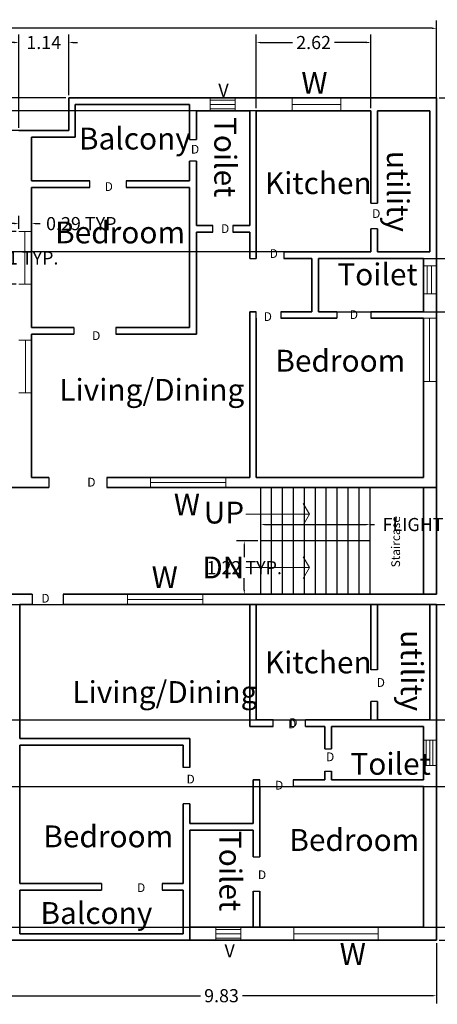
# Model space of a CAD drawing. Units: metres. Extents: x 11 to 49.6, y -23.3 to -0.8.
# Tile 4 of 5: x 25.8 to 35.3, y -23.3 to -0.8. Entities that reach past the tile are written whole.
import ezdxf

# ---------------------------------------------------------------- set-up
doc = ezdxf.new("R2010")
doc.units = ezdxf.units.M
doc.header["$MEASUREMENT"] = 0
for name, color, linetype, lineweight in [('A-ANNO-DIMS', 2, 'Continuous', 18), ('A-ANNO-IDEN', 3, 'Continuous', 18), ('A-ANNO-SYMB', 3, 'Continuous', 18), ('A-AREA-IDEN', 7, 'Continuous', 18), ('A-DOOR', 3, 'Continuous', 25), ('A-FLOR-STRS', 7, 'Continuous', 25), ('A-GLAZ', 4, 'Continuous', 18), ('A-GLAZ-VENT', 4, 'Continuous', 18), ('A-WALL', 7, 'Continuous', 35)]:
    doc.layers.add(name, color=color, linetype=linetype, lineweight=lineweight)
doc.styles.get("Standard").update_dxf_attribs({"font": 'arial.ttf'})
doc.dimstyles.get("Standard").update_dxf_attribs({"dimtxt": 0.3, "dimasz": 0.1, "dimexe": 0.18, "dimexo": 0.0625, "dimgap": 0.09, "dimtad": 0, "dimtih": 1, "dimtoh": 1, "dimzin": 0, "dimdsep": 46, "dimtxsty": 'Standard', "dimcen": 0.09, "dimadec": 0, "dimazin": 0, "dimtfac": 1, "dimtofl": 0, "dimtmove": 0, "dimatfit": 3, "dimfxl": 1, "dimtolj": 1, "dimtzin": 0, "dimarcsym": 0})

# ---------------------------------------------------------------- blocks, each defined once
blk = doc.blocks.new('*D1')
at = {"layer": 'A-ANNO-DIMS', "color": 0, "lineweight": -2, "transparency": 16777216}
for p, q in [((13.884, -3.135), (13.884, -0.816)), ((35.309, -2.864), (35.309, -0.816)), ((13.984, -0.996), (23.999, -0.996)), ((35.209, -0.996), (25.194, -0.996))]:
    blk.add_line(p, q, dxfattribs=at)
at = {"layer": 'A-ANNO-DIMS', "color": 0, "transparency": 16777216}
for points in [[(13.984, -0.979), (13.984, -1.013), (13.884, -0.996)], [(35.209, -0.979), (35.209, -1.013), (35.309, -0.996)]]:
    blk.add_solid(points, dxfattribs=at)
at = {"layer": 'Defpoints', "color": 0, "transparency": 16777216}
for p in [(35.309, -0.996), (35.309, -2.926), (13.884, -3.197)]:
    blk.add_point(p, dxfattribs=at)
at = {"layer": 'A-ANNO-DIMS', "color": 0, "transparency": 16777216, "insert": (24.597, -0.996), "char_height": 0.3, "attachment_point": 5}
blk.add_mtext('\\A1;21.42', dxfattribs=at)
blk = doc.blocks.new('WIN-1119-D300')
for p, q in [((0, 0.3), (0, 0)), ((1.119, 0.3), (1.119, 0)), ((0, 0.15), (1.119, 0.15))]:
    blk.add_line(p, q)
blk = doc.blocks.new('WIN-1207-D290')
for p, q in [((0.29, 1.207), (0, 1.207)), ((0.14, 1.207), (0.14, 0)), ((0, 0), (0.29, 0))]:
    blk.add_line(p, q)
blk = doc.blocks.new('WIN-1932-D300')
for p, q in [((0, 0.3), (0, 0)), ((1.932, 0.3), (1.932, 0)), ((1.932, 0.15), (1.932, 0.3)), ((0, 0.15), (1.932, 0.15))]:
    blk.add_line(p, q)
blk = doc.blocks.new('WIN-1724-D230')
for p, q in [((0, 0.23), (0, 0)), ((1.724, 0.23), (1.724, 0)), ((0, 0.115), (1.724, 0.115))]:
    blk.add_line(p, q)
blk = doc.blocks.new('VENT-572')
for p, q in [((0, 0.3), (0, 0)), ((0, 0.25), (0.572, 0.25)), ((0.572, 0.3), (0.572, 0)), ((0, 0.15), (0.572, 0.15)), ((0, 0.05), (0.572, 0.05))]:
    blk.add_line(p, q)
blk = doc.blocks.new('VENT-580')
for p, q in [((0, 0.58), (0.3, 0.58)), ((0.067, 0.58), (0.067, 0)), ((0.15, 0.58), (0.15, 0)), ((0.22, 0.58), (0.22, 0)), ((0, 0), (0.3, 0))]:
    blk.add_line(p, q)
blk = doc.blocks.new('DOOR-JAMB-704')
for p, q in [((0, 0.23), (0, 0)), ((0.704, 0.23), (0.704, 0))]:
    blk.add_line(p, q)
blk = doc.blocks.new('DOOR-JAMB-741')
for p, q in [((0, 0.15), (0, 0)), ((0.741, 0.15), (0.741, 0))]:
    blk.add_line(p, q)
blk = doc.blocks.new('DOOR-JAMB-721')
for p, q in [((0, 0.721), (0.15, 0.721)), ((0, 0), (0.15, 0))]:
    blk.add_line(p, q)
blk = doc.blocks.new('DOOR-JAMB-513')
for p, q in [((0, 0.513), (0.15, 0.513)), ((0, 0), (0.15, 0))]:
    blk.add_line(p, q)
blk = doc.blocks.new('DOOR-JAMB-1386')
for p, q in [((0, 0.15), (0, 0)), ((1.386, 0.15), (1.386, 0))]:
    blk.add_line(p, q)
blk = doc.blocks.new('DOOR-JAMB-789')
for p, q in [((0.15, 0.789), (0, 0.789)), ((0.15, 0), (0, 0))]:
    blk.add_line(p, q)
blk = doc.blocks.new('STAIR-DIRECTION-ARROW')
for p, q in [((1.456, 0.249), (1.313, 0.497)), ((0, 0.249), (1.456, 0.249)), ((1.456, 0.249), (1.313, 0))]:
    blk.add_line(p, q)
blk = doc.blocks.new('STAIR-FLIGHT-250-GOING')
for p, q in [((0, 0), (0, 1.22)), ((0.25, 0), (0.25, 1.22)), ((0.5, 0), (0.5, 1.22)), ((0.75, 0), (0.75, 1.22)), ((1, 0), (1, 1.22)), ((1.25, 0), (1.25, 1.22)), ((1.5, 0), (1.5, 1.22)), ((1.75, 0), (1.75, 1.22)), ((2, 0), (2, 1.22)), ((2.25, 0), (2.25, 1.22)), ((2.5, 0), (2.5, 1.22))]:
    blk.add_line(p, q)
blk = doc.blocks.new('*D36')
at = {"layer": 'A-ANNO-DIMS', "color": 0, "lineweight": -2, "transparency": 16777216}
for p, q in [((25.697, -5.642), (25.398, -5.642)), ((25.578, -5.742), (25.578, -6.005)), ((25.578, -6.749), (25.578, -6.486)), ((25.697, -6.849), (25.398, -6.849))]:
    blk.add_line(p, q, dxfattribs=at)
at = {"layer": 'A-ANNO-DIMS', "color": 0, "transparency": 16777216}
for points in [[(25.561, -5.742), (25.595, -5.742), (25.578, -5.642)], [(25.561, -6.749), (25.595, -6.749), (25.578, -6.849)]]:
    blk.add_solid(points, dxfattribs=at)
at = {"layer": 'Defpoints', "color": 0, "transparency": 16777216}
for p in [(25.578, -5.642), (25.759, -5.642), (25.759, -6.849)]:
    blk.add_point(p, dxfattribs=at)
at = {"layer": 'A-ANNO-DIMS', "color": 0, "transparency": 16777216, "insert": (25.578, -6.246), "char_height": 0.3, "attachment_point": 5}
blk.add_mtext('\\A1;W 1.21 TYP.', dxfattribs=at)
blk = doc.blocks.new('*D37')
at = {"layer": 'A-ANNO-DIMS', "color": 0, "lineweight": -2, "transparency": 16777216}
for p, q in [((25.759, -5.579), (25.759, -5.281)), ((26.05, -5.579), (26.05, -5.281)), ((25.659, -5.461), (25.559, -5.461)), ((26.15, -5.461), (26.25, -5.461))]:
    blk.add_line(p, q, dxfattribs=at)
at = {"layer": 'A-ANNO-DIMS', "color": 0, "transparency": 16777216}
for points in [[(25.659, -5.444), (25.659, -5.477), (25.759, -5.461)], [(26.15, -5.444), (26.15, -5.477), (26.05, -5.461)]]:
    blk.add_solid(points, dxfattribs=at)
at = {"layer": 'Defpoints', "color": 0, "transparency": 16777216}
for p in [(26.05, -5.461), (25.759, -5.642), (26.05, -5.642)]:
    blk.add_point(p, dxfattribs=at)
at = {"layer": 'A-ANNO-DIMS', "color": 0, "transparency": 16777216, "insert": (27.244, -5.461), "char_height": 0.3, "attachment_point": 5}
blk.add_mtext('\\A1;0.29 TYP.', dxfattribs=at)
blk = doc.blocks.new('*D54')
at = {"layer": 'A-ANNO-DIMS', "color": 0, "lineweight": -2, "transparency": 16777216}
for p, q in [((31.289, -12.654), (31.289, -12.161)), ((31.389, -12.341), (33.689, -12.341)), ((33.789, -12.654), (33.789, -12.161)), ((33.789, -12.341), (33.889, -12.341))]:
    blk.add_line(p, q, dxfattribs=at)
at = {"layer": 'A-ANNO-DIMS', "color": 0, "transparency": 16777216}
for points in [[(31.389, -12.324), (31.389, -12.358), (31.289, -12.341)], [(33.689, -12.324), (33.689, -12.358), (33.789, -12.341)]]:
    blk.add_solid(points, dxfattribs=at)
at = {"layer": 'Defpoints', "color": 0, "transparency": 16777216}
for p in [(33.789, -12.341), (31.289, -12.716), (33.789, -12.716)]:
    blk.add_point(p, dxfattribs=at)
at = {"layer": 'A-ANNO-DIMS', "color": 0, "transparency": 16777216, "insert": (35.679, -12.341), "char_height": 0.3, "attachment_point": 5}
blk.add_mtext('\\A1;FLIGHT 2.50 TYP.', dxfattribs=at)
blk = doc.blocks.new('*D55')
at = {"layer": 'A-ANNO-DIMS', "color": 0, "lineweight": -2, "transparency": 16777216}
for p, q in [((31.227, -12.716), (30.734, -12.716)), ((30.914, -12.816), (30.914, -13.085)), ((30.914, -13.836), (30.914, -13.567)), ((31.227, -13.936), (30.734, -13.936))]:
    blk.add_line(p, q, dxfattribs=at)
at = {"layer": 'A-ANNO-DIMS', "color": 0, "transparency": 16777216}
for points in [[(30.898, -12.816), (30.931, -12.816), (30.914, -12.716)], [(30.898, -13.836), (30.931, -13.836), (30.914, -13.936)]]:
    blk.add_solid(points, dxfattribs=at)
at = {"layer": 'Defpoints', "color": 0, "transparency": 16777216}
for p in [(30.914, -12.716), (31.289, -12.716), (31.289, -13.936)]:
    blk.add_point(p, dxfattribs=at)
at = {"layer": 'A-ANNO-DIMS', "color": 0, "transparency": 16777216, "insert": (30.914, -13.326), "char_height": 0.3, "attachment_point": 5}
blk.add_mtext('\\A1;1.22 TYP.', dxfattribs=at)
blk = doc.blocks.new('*D56')
at = {"layer": 'A-ANNO-DIMS', "color": 0, "lineweight": -2, "transparency": 16777216}
for p, q in [((35.372, -2.586), (36.754, -2.586)), ((36.574, -2.686), (36.574, -11.973)), ((36.574, -21.746), (36.574, -12.459)), ((35.372, -21.846), (36.754, -21.846))]:
    blk.add_line(p, q, dxfattribs=at)
at = {"layer": 'A-ANNO-DIMS', "color": 0, "transparency": 16777216}
for points in [[(36.558, -2.686), (36.591, -2.686), (36.574, -2.586)], [(36.558, -21.746), (36.591, -21.746), (36.574, -21.846)]]:
    blk.add_solid(points, dxfattribs=at)
at = {"layer": 'Defpoints', "color": 0, "transparency": 16777216}
for p in [(35.309, -2.586), (35.309, -21.846), (36.574, -21.846)]:
    blk.add_point(p, dxfattribs=at)
at = {"layer": 'A-ANNO-DIMS', "color": 0, "transparency": 16777216, "insert": (36.574, -12.216), "char_height": 0.3, "attachment_point": 5}
blk.add_mtext('\\A1;19.26', dxfattribs=at)
blk = doc.blocks.new('*D57')
at = {"layer": 'A-ANNO-DIMS', "color": 0, "lineweight": -2, "transparency": 16777216}
for p, q in [((33.747, -2.886), (12.454, -2.886)), ((12.634, -2.986), (12.634, -4.253)), ((12.634, -6.006), (12.634, -4.739)), ((33.747, -6.106), (12.454, -6.106))]:
    blk.add_line(p, q, dxfattribs=at)
at = {"layer": 'A-ANNO-DIMS', "color": 0, "transparency": 16777216}
for points in [[(12.618, -2.986), (12.651, -2.986), (12.634, -2.886)], [(12.618, -6.006), (12.651, -6.006), (12.634, -6.106)]]:
    blk.add_solid(points, dxfattribs=at)
at = {"layer": 'Defpoints', "color": 0, "transparency": 16777216}
for p in [(33.809, -2.886), (12.634, -6.106), (33.809, -6.106)]:
    blk.add_point(p, dxfattribs=at)
at = {"layer": 'A-ANNO-DIMS', "color": 0, "transparency": 16777216, "insert": (12.634, -4.496), "char_height": 0.3, "attachment_point": 5}
blk.add_mtext('\\A1;3.22', dxfattribs=at)
blk = doc.blocks.new('*D58')
at = {"layer": 'A-ANNO-DIMS', "color": 0, "lineweight": -2, "transparency": 16777216}
for p, q in [((32.672, -6.256), (36.754, -6.256)), ((36.574, -6.356), (36.574, -6.625)), ((36.574, -7.376), (36.574, -7.107)), ((32.672, -7.476), (36.754, -7.476))]:
    blk.add_line(p, q, dxfattribs=at)
at = {"layer": 'A-ANNO-DIMS', "color": 0, "transparency": 16777216}
for points in [[(36.558, -6.356), (36.591, -6.356), (36.574, -6.256)], [(36.558, -7.376), (36.591, -7.376), (36.574, -7.476)]]:
    blk.add_solid(points, dxfattribs=at)
at = {"layer": 'Defpoints', "color": 0, "transparency": 16777216}
for p in [(32.609, -6.256), (32.609, -7.476), (36.574, -7.476)]:
    blk.add_point(p, dxfattribs=at)
at = {"layer": 'A-ANNO-DIMS', "color": 0, "transparency": 16777216, "insert": (36.574, -6.866), "char_height": 0.3, "attachment_point": 5}
blk.add_mtext('\\A1;1.22', dxfattribs=at)
blk = doc.blocks.new('*D59')
at = {"layer": 'A-ANNO-DIMS', "color": 0, "lineweight": -2, "transparency": 16777216}
for p, q in [((31.189, -2.824), (31.189, -1.141)), ((31.289, -1.321), (32.019, -1.321)), ((33.709, -1.321), (32.98, -1.321)), ((33.809, -2.824), (33.809, -1.141))]:
    blk.add_line(p, q, dxfattribs=at)
at = {"layer": 'A-ANNO-DIMS', "color": 0, "transparency": 16777216}
for points in [[(31.289, -1.304), (31.289, -1.338), (31.189, -1.321)], [(33.709, -1.304), (33.709, -1.338), (33.809, -1.321)]]:
    blk.add_solid(points, dxfattribs=at)
at = {"layer": 'Defpoints', "color": 0, "transparency": 16777216}
for p in [(33.809, -1.321), (31.189, -2.886), (33.809, -2.886)]:
    blk.add_point(p, dxfattribs=at)
at = {"layer": 'A-ANNO-DIMS', "color": 0, "transparency": 16777216, "insert": (32.499, -1.321), "char_height": 0.3, "attachment_point": 5}
blk.add_mtext('\\A1;2.62', dxfattribs=at)
blk = doc.blocks.new('*D61')
at = {"layer": 'A-ANNO-DIMS', "color": 0, "lineweight": -2, "transparency": 16777216}
for p, q in [((25.659, -1.321), (25.559, -1.321)), ((25.759, -3.274), (25.759, -1.141)), ((26.9, -2.524), (26.9, -1.141)), ((27, -1.321), (27.1, -1.321))]:
    blk.add_line(p, q, dxfattribs=at)
at = {"layer": 'A-ANNO-DIMS', "color": 0, "transparency": 16777216}
for points in [[(25.659, -1.304), (25.659, -1.338), (25.759, -1.321)], [(27, -1.304), (27, -1.338), (26.9, -1.321)]]:
    blk.add_solid(points, dxfattribs=at)
at = {"layer": 'Defpoints', "color": 0, "transparency": 16777216}
for p in [(25.759, -1.321), (26.9, -2.586), (25.759, -3.336)]:
    blk.add_point(p, dxfattribs=at)
at = {"layer": 'A-ANNO-DIMS', "color": 0, "transparency": 16777216, "insert": (26.329, -1.321), "char_height": 0.3, "attachment_point": 5}
blk.add_mtext('\\A1;1.14', dxfattribs=at)
blk = doc.blocks.new('*D62')
at = {"layer": 'A-ANNO-DIMS', "color": 0, "lineweight": -2, "transparency": 16777216}
for p, q in [((12.634, -2.486), (12.634, -2.386)), ((26.837, -2.586), (12.454, -2.586)), ((26.837, -3.336), (12.454, -3.336)), ((12.634, -3.436), (12.634, -3.536))]:
    blk.add_line(p, q, dxfattribs=at)
at = {"layer": 'A-ANNO-DIMS', "color": 0, "transparency": 16777216}
for points in [[(12.618, -2.486), (12.651, -2.486), (12.634, -2.586)], [(12.618, -3.436), (12.651, -3.436), (12.634, -3.336)]]:
    blk.add_solid(points, dxfattribs=at)
at = {"layer": 'Defpoints', "color": 0, "transparency": 16777216}
for p in [(26.9, -2.586), (12.634, -3.336), (26.9, -3.336)]:
    blk.add_point(p, dxfattribs=at)
at = {"layer": 'A-ANNO-DIMS', "color": 0, "transparency": 16777216, "insert": (12.634, -2.961), "char_height": 0.3, "attachment_point": 5}
blk.add_mtext('\\A1;0.75', dxfattribs=at)
blk = doc.blocks.new('*D64')
at = {"layer": 'A-ANNO-DIMS', "color": 0, "lineweight": -2, "transparency": 16777216}
for p, q in [((25.48, -21.909), (25.48, -23.292)), ((35.309, -21.909), (35.309, -23.292)), ((25.58, -23.112), (29.915, -23.112)), ((35.209, -23.112), (30.874, -23.112))]:
    blk.add_line(p, q, dxfattribs=at)
at = {"layer": 'A-ANNO-DIMS', "color": 0, "transparency": 16777216}
for points in [[(25.58, -23.096), (25.58, -23.129), (25.48, -23.112)], [(35.209, -23.096), (35.209, -23.129), (35.309, -23.112)]]:
    blk.add_solid(points, dxfattribs=at)
at = {"layer": 'Defpoints', "color": 0, "transparency": 16777216}
for p in [(25.48, -21.846), (35.309, -21.846), (35.309, -23.112)]:
    blk.add_point(p, dxfattribs=at)
at = {"layer": 'A-ANNO-DIMS', "color": 0, "transparency": 16777216, "insert": (30.394, -23.112), "char_height": 0.3, "attachment_point": 5}
blk.add_mtext('\\A1;9.83', dxfattribs=at)
blk = doc.blocks.new('*D71')
at = {"layer": 'A-ANNO-DIMS', "color": 0, "lineweight": -2, "transparency": 16777216}
for p, q in [((23.641, -14.166), (36.754, -14.166)), ((36.574, -14.266), (36.574, -15.243)), ((36.574, -16.706), (36.574, -15.729)), ((23.641, -16.806), (36.754, -16.806))]:
    blk.add_line(p, q, dxfattribs=at)
at = {"layer": 'A-ANNO-DIMS', "color": 0, "transparency": 16777216}
for points in [[(36.558, -14.266), (36.591, -14.266), (36.574, -14.166)], [(36.558, -16.706), (36.591, -16.706), (36.574, -16.806)]]:
    blk.add_solid(points, dxfattribs=at)
at = {"layer": 'Defpoints', "color": 0, "transparency": 16777216}
for p in [(23.579, -14.166), (23.579, -16.806), (36.574, -16.806)]:
    blk.add_point(p, dxfattribs=at)
at = {"layer": 'A-ANNO-DIMS', "color": 0, "transparency": 16777216, "insert": (36.574, -15.486), "char_height": 0.3, "attachment_point": 5}
blk.add_mtext('\\A1;2.64', dxfattribs=at)
blk = doc.blocks.new('*D72')
at = {"layer": 'A-ANNO-DIMS', "color": 0, "lineweight": -2, "transparency": 16777216}
for p, q in [((23.491, -18.326), (36.754, -18.326)), ((36.574, -18.426), (36.574, -19.693)), ((36.574, -21.446), (36.574, -20.179)), ((23.491, -21.546), (36.754, -21.546))]:
    blk.add_line(p, q, dxfattribs=at)
at = {"layer": 'A-ANNO-DIMS', "color": 0, "transparency": 16777216}
for points in [[(36.558, -18.426), (36.591, -18.426), (36.574, -18.326)], [(36.558, -21.446), (36.591, -21.446), (36.574, -21.546)]]:
    blk.add_solid(points, dxfattribs=at)
at = {"layer": 'Defpoints', "color": 0, "transparency": 16777216}
for p in [(23.429, -18.326), (23.429, -21.546), (36.574, -21.546)]:
    blk.add_point(p, dxfattribs=at)
at = {"layer": 'A-ANNO-DIMS', "color": 0, "transparency": 16777216, "insert": (36.574, -19.936), "char_height": 0.3, "attachment_point": 5}
blk.add_mtext('\\A1;3.22', dxfattribs=at)

msp = doc.modelspace()

# ---------------------------------------------------------------- linework, layer by layer
at = {"layer": 'A-DOOR'}
for p, q in [((29.66, -3.541), (29.819, -3.541)), ((29.819, -4.035), (29.66, -4.035)), ((27.38, -4.636), (27.38, -4.486)), ((28.217, -4.486), (28.217, -4.636)), ((33.809, -4.992), (33.959, -4.992)), ((30.194, -5.656), (30.194, -5.506)), ((30.651, -5.506), (30.651, -5.656)), ((33.959, -5.58), (33.809, -5.58)), ((31.039, -6.256), (31.189, -6.256)), ((31.819, -6.106), (31.819, -6.256)), ((31.189, -7.626), (31.189, -7.476)), ((31.749, -7.476), (31.749, -7.626)), ((33.031, -7.476), (33.031, -7.626)), ((33.809, -7.476), (33.809, -7.626)), ((27.017, -7.836), (27.017, -7.987)), ((27.976, -7.836), (27.976, -7.987)), ((26.444, -11.266), (26.444, -11.496)), ((27.774, -11.266), (27.774, -11.496)), ((29.669, -17.893), (29.519, -17.893)), ((31.269, -18.326), (31.269, -18.176)), ((32.028, -18.176), (32.028, -18.326)), ((29.669, -18.729), (29.519, -18.729))]:
    msp.add_line(p, q, dxfattribs=at)
at = {"layer": 'A-FLOR-STRS'}
msp.add_line((33.789, -12.716), (31.289, -12.716), dxfattribs=at)
at = {"layer": 'A-GLAZ'}
for p, q in [((35.009, -7.626), (35.309, -7.626)), ((35.147, -7.626), (35.147, -9.069)), ((35.309, -9.069), (35.009, -9.069))]:
    msp.add_line(p, q, dxfattribs=at)
at = {"layer": 'A-GLAZ-VENT'}
for p, q in [((35.009, -6.426), (35.309, -6.426)), ((35.094, -6.426), (35.094, -7.067)), ((35.094, -6.426), (35.094, -7.067)), ((35.094, -6.426), (35.094, -7.067)), ((35.194, -6.426), (35.194, -7.067)), ((35.009, -7.067), (35.309, -7.067))]:
    msp.add_line(p, q, dxfattribs=at)
at = {"layer": 'A-WALL'}
for p, q in [((26.9, -2.586), (35.309, -2.586)), ((26.9, -2.586), (26.9, -3.336)), ((35.309, -2.586), (35.309, -13.936)), ((27.05, -2.736), (29.66, -2.736)), ((27.05, -2.736), (27.05, -3.486)), ((29.66, -2.736), (29.66, -3.541)), ((29.819, -2.886), (29.819, -3.541)), ((29.819, -2.886), (31.039, -2.886)), ((31.039, -2.886), (31.039, -5.506)), ((31.189, -2.886), (31.189, -6.106)), ((31.189, -2.886), (33.809, -2.886)), ((33.809, -2.886), (33.809, -4.992)), ((33.959, -2.886), (33.959, -4.992)), ((33.959, -2.886), (35.159, -2.886)), ((35.159, -2.886), (35.159, -6.106)), ((25.759, -3.336), (26.9, -3.336)), ((26.05, -3.486), (26.05, -4.486)), ((26.05, -3.486), (27.05, -3.486)), ((29.66, -4.035), (29.66, -4.486)), ((29.819, -4.035), (29.819, -5.506)), ((26.05, -4.486), (27.38, -4.486)), ((28.217, -4.486), (29.66, -4.486)), ((26.05, -4.636), (27.38, -4.636)), ((26.05, -4.636), (26.05, -7.836)), ((28.217, -4.636), (29.66, -4.636)), ((29.66, -4.636), (29.66, -7.836)), ((29.819, -5.506), (30.194, -5.506)), ((30.651, -5.506), (31.039, -5.506)), ((33.809, -5.58), (33.809, -6.106)), ((33.959, -5.58), (33.959, -6.106)), ((29.819, -5.656), (30.194, -5.656)), ((29.819, -5.656), (29.819, -7.987)), ((30.651, -5.656), (31.039, -5.656)), ((31.039, -5.656), (31.039, -6.256)), ((31.189, -5.656), (31.189, -6.256)), ((31.819, -6.106), (33.809, -6.106)), ((31.819, -6.256), (32.459, -6.256)), ((32.459, -6.256), (32.459, -7.476)), ((32.609, -6.256), (32.609, -7.476)), ((32.609, -6.256), (35.009, -6.256)), ((33.959, -6.106), (35.159, -6.106)), ((35.009, -6.256), (35.009, -7.476)), ((29.819, -6.406), (29.819, -7.987)), ((31.039, -7.476), (31.189, -7.476)), ((31.039, -7.476), (31.039, -11.266)), ((31.039, -7.626), (31.039, -11.266)), ((31.189, -7.626), (31.189, -11.266)), ((31.749, -7.476), (32.459, -7.476)), ((31.749, -7.626), (33.031, -7.626)), ((32.609, -7.476), (33.031, -7.476)), ((33.809, -7.476), (35.009, -7.476)), ((33.809, -7.626), (35.009, -7.626)), ((35.009, -7.626), (35.009, -11.266)), ((26.05, -7.836), (27.017, -7.836)), ((27.976, -7.836), (29.66, -7.836)), ((26.05, -7.987), (27.017, -7.987)), ((26.05, -7.987), (26.05, -11.266)), ((27.976, -7.987), (29.819, -7.987)), ((26.05, -11.266), (26.444, -11.266)), ((27.774, -11.266), (31.039, -11.266)), ((31.189, -11.266), (35.009, -11.266)), ((15.505, -11.496), (26.444, -11.496)), ((15.505, -11.496), (26.444, -11.496)), ((27.774, -11.496), (35.009, -11.496)), ((27.774, -11.496), (35.009, -11.496)), ((35.009, -11.496), (35.009, -13.936)), ((35.009, -11.496), (35.309, -11.496)), ((35.009, -12.716), (35.009, -11.496)), ((35.009, -13.936), (35.009, -12.716)), ((15.36, -13.936), (26.068, -13.936)), ((15.36, -13.936), (26.068, -13.936)), ((26.772, -13.936), (35.009, -13.936)), ((26.772, -13.936), (35.009, -13.936)), ((35.009, -13.936), (35.309, -13.936)), ((25.78, -14.166), (25.78, -17.236)), ((25.78, -14.166), (26.068, -14.166)), ((26.772, -14.166), (30.989, -14.166)), ((26.772, -14.166), (31.039, -14.166)), ((31.039, -16.806), (31.039, -14.166)), ((31.039, -16.956), (31.039, -14.166)), ((31.039, -14.166), (31.689, -14.166)), ((31.189, -16.806), (31.189, -14.166)), ((31.439, -14.166), (32.549, -14.166)), ((31.539, -14.166), (33.809, -14.166)), ((32.249, -14.166), (33.759, -14.166)), ((33.809, -14.166), (35.259, -14.166)), ((33.809, -15.662), (33.809, -14.166)), ((33.959, -15.662), (33.959, -14.166)), ((34.209, -14.166), (35.309, -14.166)), ((35.159, -16.806), (35.159, -14.166)), ((35.309, -21.846), (35.309, -14.166)), ((33.809, -16.806), (33.809, -16.383)), ((33.959, -16.806), (33.959, -16.383)), ((31.189, -16.806), (31.576, -16.806)), ((32.317, -16.806), (33.809, -16.806)), ((33.959, -16.806), (35.159, -16.806)), ((31.039, -16.956), (31.576, -16.956)), ((32.317, -16.956), (32.759, -16.956)), ((32.759, -17.468), (32.759, -16.956)), ((32.909, -16.956), (35.009, -16.956)), ((32.909, -17.468), (32.909, -16.956)), ((35.009, -18.176), (35.009, -16.956)), ((25.78, -17.236), (29.669, -17.236)), ((29.669, -17.893), (29.669, -17.236)), ((25.78, -17.386), (25.78, -20.546)), ((25.78, -17.386), (29.519, -17.386)), ((29.519, -17.893), (29.519, -17.386)), ((32.759, -18.176), (32.759, -17.981)), ((32.909, -18.176), (32.909, -17.981)), ((35.009, -18.176), (35.009, -17.926)), ((31.119, -18.176), (31.269, -18.176)), ((31.119, -19.176), (31.119, -18.176)), ((32.028, -18.176), (32.759, -18.176)), ((32.909, -18.176), (35.009, -18.176)), ((31.269, -19.936), (31.269, -18.326)), ((32.028, -18.326), (35.009, -18.326)), ((35.009, -21.546), (35.009, -18.326)), ((29.519, -20.546), (29.519, -18.729)), ((29.669, -19.176), (29.669, -18.729)), ((29.669, -19.176), (31.119, -19.176)), ((29.669, -19.326), (31.119, -19.326)), ((29.669, -21.846), (29.669, -19.326)), ((31.119, -19.376), (31.119, -19.326)), ((31.119, -19.936), (31.119, -19.326)), ((25.78, -20.546), (27.651, -20.546)), ((25.78, -20.696), (25.78, -21.696)), ((25.78, -20.696), (27.651, -20.696)), ((29.037, -20.546), (29.519, -20.546)), ((29.037, -20.696), (29.519, -20.696)), ((29.519, -21.696), (29.519, -20.696)), ((31.119, -21.546), (31.119, -20.725)), ((31.269, -21.546), (31.269, -20.725)), ((29.669, -21.546), (31.269, -21.546)), ((31.119, -21.546), (35.009, -21.546)), ((25.78, -21.696), (29.519, -21.696)), ((25.48, -21.846), (35.309, -21.846))]:
    msp.add_line(p, q, dxfattribs=at)

# ---------------------------------------------------------------- block references
at = {"layer": 'A-ANNO-SYMB'}
for p in [(30.947, -12.355), (30.947, -13.575)]:
    msp.add_blockref('STAIR-DIRECTION-ARROW', p, dxfattribs=at)
at = {"layer": 'A-DOOR'}
for name, p in [('DOOR-JAMB-704', (26.068, -14.166)), ('DOOR-JAMB-513', (32.759, -17.981)), ('DOOR-JAMB-1386', (27.651, -20.696))]:
    msp.add_blockref(name, p, dxfattribs=at)
at = {"layer": 'A-DOOR', "rotation": 180}
for name, p in [('DOOR-JAMB-721', (33.959, -15.662)), ('DOOR-JAMB-741', (32.317, -16.806)), ('DOOR-JAMB-789', (31.269, -19.936))]:
    msp.add_blockref(name, p, dxfattribs=at)
at = {"layer": 'A-FLOR-STRS'}
for p in [(31.289, -12.716), (31.289, -13.936)]:
    msp.add_blockref('STAIR-FLIGHT-250-GOING', p, dxfattribs=at)
at = {"layer": 'A-GLAZ'}
for name, p in [('WIN-1119-D300', (32.006, -2.886)), ('WIN-1207-D290', (25.759, -6.849)), ('WIN-1724-D230', (28.771, -11.496)), ('WIN-1724-D230', (28.245, -14.166)), ('WIN-1932-D300', (32.046, -21.846))]:
    msp.add_blockref(name, p, dxfattribs=at)
at = {"layer": 'A-GLAZ', "rotation": 180}
msp.add_blockref('WIN-1207-D290', (26.05, -8.123), dxfattribs=at)
at = {"layer": 'A-GLAZ-VENT'}
for name, p in [('VENT-572', (30.132, -2.886)), ('VENT-580', (35.007, -17.853)), ('VENT-572', (30.26, -21.847))]:
    msp.add_blockref(name, p, dxfattribs=at)

# ---------------------------------------------------------------- texts
at = {"layer": 'A-ANNO-IDEN', "attachment_point": 1}
for s, width, insert, char_height in [('W', 1.41386, (32.218, -1.993), 0.5), ('V', 0.1, (30.321, -2.265), 0.3), ('D', 0.77129, (29.695, -3.661), 0.2), ('D', 0.77129, (27.722, -4.515), 0.2), ('D', 0.77129, (33.838, -5.131), 0.2), ('D', 0.77129, (30.382, -5.476), 0.2), ('D', 0.77129, (31.494, -6.046), 0.2), ('D', 0.77129, (31.358, -7.487), 0.2), ('D', 0.77129, (33.327, -7.442), 0.2), ('D', 0.77129, (27.436, -7.922), 0.2), ('D', 0.77129, (27.325, -11.272), 0.2), ('W', 1.41386, (29.303, -11.634), 0.5), ('W', 1.41386, (28.796, -13.295), 0.5), ('D', 0.77129, (26.275, -13.926), 0.2), ('D', 0.77129, (33.942, -15.852), 0.2), ('D', 0.77129, (31.913, -16.799), 0.2), ('D', 0.77129, (31.942, -16.77), 0.2), ('D', 0.77129, (32.784, -17.551), 0.2), ('D', 0.77129, (32.784, -17.551), 0.2), ('D', 0.77129, (29.594, -18.061), 0.2), ('D', 0.77129, (31.617, -18.2), 0.2), ('D', 0.77129, (31.226, -20.248), 0.2), ('D', 0.77129, (28.462, -20.542), 0.2), ('V', 0.1, (30.462, -21.935), 0.3), ('W', 1.41386, (33.095, -21.911), 0.5)]:
    msp.add_mtext_dynamic_manual_height_columns(s, width=width, gutter_width=0.5, heights=[0], dxfattribs=dict(at, insert=insert, char_height=char_height))
at = {"layer": 'A-ANNO-SYMB'}
for s, p in [('UP', (29.988, -12.317)), ('DN', (29.954, -13.572))]:
    msp.add_text(s, height=0.5, dxfattribs=at).set_placement(p)
at = {"layer": 'A-AREA-IDEN'}
msp.add_text('Staircase', height=0.2, rotation=90, dxfattribs=at).set_placement((34.475, -13.32))
at = {"layer": 'A-AREA-IDEN', "char_height": 0.5, "rotation": 270}
for s, insert, attachment_point in [('Toilet', (30.73, -3.023), 1), ('utility', (34.676, -3.799), 1), ('utility', (34.996, -14.755), 1), ('Toilet', (30.847, -21.182), 3)]:
    msp.add_mtext_dynamic_manual_height_columns(s, width=2.63335, gutter_width=1, heights=[0], dxfattribs=dict(at, insert=insert, attachment_point=attachment_point))
at = {"layer": 'A-AREA-IDEN', "char_height": 0.5}
for s, insert, attachment_point in [('Balcony', (27.134, -3.267), 1), ('Kitchen', (31.385, -4.286), 1), ('Bedroom', (26.589, -5.413), 1), ('Toilet', (33.041, -6.371), 1), ('Bedroom', (31.624, -8.346), 1), ('Living/Dining', (26.684, -9.011), 1), ('Kitchen', (31.385, -15.243), 1), ('Living/Dining', (26.984, -16.421), 7), ('Toilet', (33.341, -18.061), 7), ('Bedroom', (26.319, -19.72), 7), ('Bedroom', (31.944, -19.302), 1), ('Balcony', (26.254, -21.472), 7)]:
    msp.add_mtext_dynamic_manual_height_columns(s, width=2.63335, gutter_width=1, heights=[0], dxfattribs=dict(at, insert=insert, attachment_point=attachment_point))

# ---------------------------------------------------------------- dimensions: what is measured, and where the dimension line sits
at = {"layer": 'A-ANNO-DIMS'}
for base, p1, p2, override, picture, middle in [((35.3087, -0.9961), (13.8844, -3.197), (35.3087, -2.9263), {"dimclrd": 0, "dimclre": 0, "dimclrt": 0}, '*D1', (24.5966, -0.9961)), ((25.759, -1.321), (26.9, -2.586), (25.759, -3.336), {"dimdec": 2, "dimlfac": 1, "dimrnd": 0, "dimzin": 0, "dimdsep": 46, "dimlunit": 2}, '*D61', (26.329, -1.321)), ((33.809, -1.321), (31.189, -2.886), (33.809, -2.886), {"dimdec": 2, "dimlfac": 1, "dimrnd": 0, "dimzin": 0, "dimdsep": 46, "dimlunit": 2}, '*D59', (32.499, -1.321)), ((35.309, -23.112), (25.48, -21.846), (35.309, -21.846), {"dimdec": 2, "dimlfac": 1, "dimrnd": 0, "dimzin": 0, "dimdsep": 46, "dimlunit": 2}, '*D64', (30.394, -23.112))]:
    dim = msp.add_linear_dim(base=base, p1=p1, p2=p2, dimstyle='Standard', override=override, dxfattribs=at)
    dim.commit()
    dim.dimension.update_dxf_attribs({"geometry": picture, "text_midpoint": middle})
for base, p1, p2, picture, middle in [((12.634, -3.336), (26.9, -2.586), (26.9, -3.336), '*D62', (12.634, -2.961)), ((36.574, -21.846), (35.309, -2.586), (35.309, -21.846), '*D56', (36.574, -12.216)), ((12.634, -6.106), (33.809, -2.886), (33.809, -6.106), '*D57', (12.634, -4.496)), ((36.574, -7.476), (32.609, -6.256), (32.609, -7.476), '*D58', (36.574, -6.866)), ((36.574, -16.806), (23.579, -14.166), (23.579, -16.806), '*D71', (36.574, -15.486)), ((36.574, -21.546), (23.429, -18.326), (23.429, -21.546), '*D72', (36.574, -19.936))]:
    dim = msp.add_linear_dim(base=base, p1=p1, p2=p2, angle=90, dimstyle='Standard', override={"dimdec": 2, "dimlfac": 1, "dimrnd": 0, "dimzin": 0, "dimdsep": 46, "dimlunit": 2}, dxfattribs=at)
    dim.commit()
    dim.dimension.update_dxf_attribs({"geometry": picture, "text_midpoint": middle})
for base, p1, p2, text, picture, middle in [((26.05, -5.461), (25.759, -5.642), (26.05, -5.642), '<> TYP.', '*D37', (27.244, -5.461)), ((33.789, -12.341), (31.289, -12.716), (33.789, -12.716), 'FLIGHT <> TYP.', '*D54', (35.679, -12.341))]:
    dim = msp.add_linear_dim(base=base, p1=p1, p2=p2, text=text, dimstyle='Standard', override={"dimdec": 2, "dimlfac": 1, "dimrnd": 0, "dimzin": 0, "dimdsep": 46, "dimlunit": 2}, dxfattribs=at)
    dim.commit()
    dim.dimension.update_dxf_attribs({"geometry": picture, "text_midpoint": middle})
for base, p1, p2, text, picture, middle in [((25.578, -5.642), (25.759, -6.849), (25.759, -5.642), 'W <> TYP.', '*D36', (25.578, -6.246)), ((30.914, -12.716), (31.289, -13.936), (31.289, -12.716), '<> TYP.', '*D55', (30.914, -13.326))]:
    dim = msp.add_linear_dim(base=base, p1=p1, p2=p2, angle=90, text=text, dimstyle='Standard', override={"dimdec": 2, "dimlfac": 1, "dimrnd": 0, "dimzin": 0, "dimdsep": 46, "dimlunit": 2}, dxfattribs=at)
    dim.commit()
    dim.dimension.update_dxf_attribs({"geometry": picture, "text_midpoint": middle})

doc.saveas('drawing.dxf')
